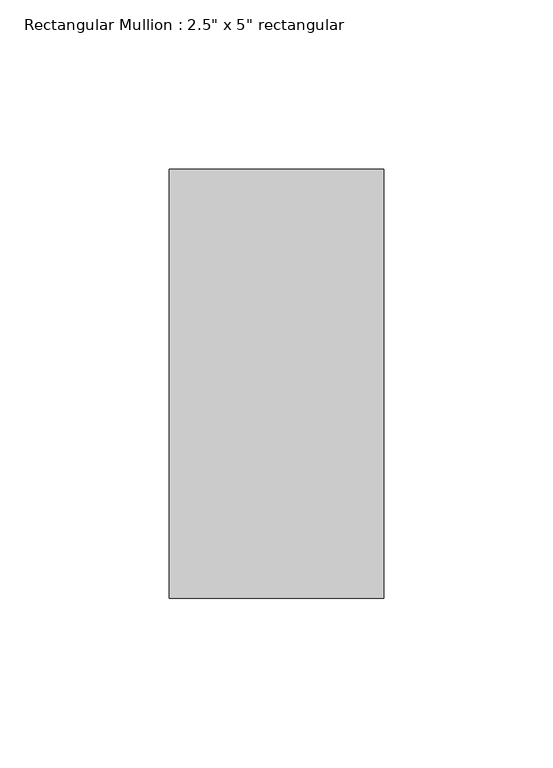
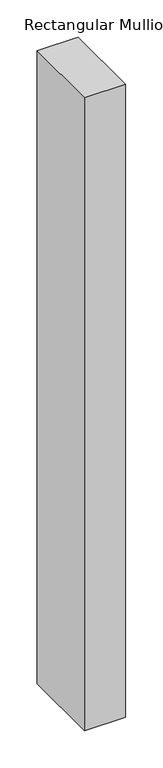
"""IFC4 building model written with IfcOpenShell, lengths in millimetres: member geometry."""

from ifc_helpers import new_model, si_unit, frame, origin, place, context, project, spatial, polyline, outline, extrude, source, transform, mapped, element, save


def member_309cb93c(model_context):
    return source(origin(), model_context, "Body", "SweptSolid", [
        extrude(outline(polyline([(31.75, 63.5), (31.75, -63.5), (-31.75, -63.5), (-31.75, 63.5), (31.75, 63.5)])), frame((0.0, 0.0, -1035.05), z_axis=(0.0, 0.0, 1.0), x_axis=(1.0, 0.0, 0.0)), (0.0, 0.0, 1.0), 1035.05),
    ])


if __name__ == "__main__":
    model = new_model("IFC4")
    model_context = context("Model", 3, world=origin())
    ifc_project = project(units=[si_unit("LENGTHUNIT", "METRE", prefix="MILLI")], contexts=[model_context])
    site = spatial("IfcSite", under=ifc_project)
    building = spatial("IfcBuilding", under=site)
    placement = place(None, origin())
    member_shape = member_309cb93c(model_context)
    element("IfcMember", 1, ObjectType="Rectangular Mullion : 2.5\" x 5\" rectangular", at=placement, inside=building, context=model_context, shape_type="MappedRepresentation", body=[
        mapped(member_shape, transform((0.0, 0.0, 0.0), x_axis=(1.0, 0.0, 0.0), y_axis=(0.0, 1.0, 0.0), z_axis=(0.0, 0.0, 1.0))),
    ])
    save(model, "model.ifc")

# Revit data of these elements
# Type "Rectangular Mullion : 2.5\" x 5\" rectangular"
#   built-in parameter 1007304 = 0.416667 (stored number, unit not read)
#   built-in parameter 1007301 = 0.104167 (stored number, unit not read)
#   built-in parameter 1007300 = 0.104167 (stored number, unit not read)
# Element 1 (IfcMember, "Rectangular Mullion : 2.5\" x 5\" rectangular")
#   Materials on its faces: "metal black"
# Materials
#   "metal black": class "Generic", colour RGB 120 120 120, transparency 0, Cost = 0
